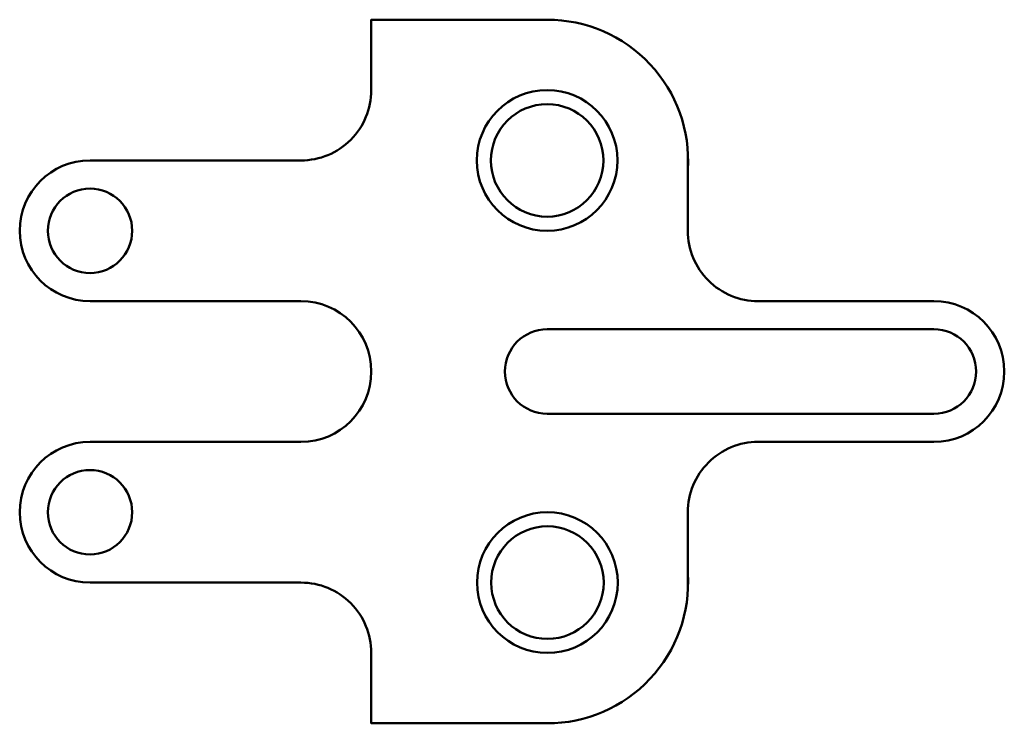
# Model space of a CAD drawing. Units: inches. Extents: x 1100 to 1240, y 1123 to 1223.
import ezdxf

# ---------------------------------------------------------------- set-up
doc = ezdxf.new("R2010")
doc.units = ezdxf.units.IN
doc.header["$MEASUREMENT"] = 0
doc.layers.add('M-OUTL', color=7, linetype='Continuous', lineweight=50)

# ---------------------------------------------------------------- blocks, each defined once
blk = doc.blocks.new('HOLE-CBORE-D16')
for radius in [10, 8]:
    blk.add_circle((1174.65, 1203.2, 23), radius)

msp = doc.modelspace()

# ---------------------------------------------------------------- linework, layer by layer
at = {"layer": 'M-OUTL', "extrusion": (0, 1, 0)}
msp.add_line((1109.65, 1203.2), (1124.65, 1203.2), dxfattribs=at)
at = {"layer": 'M-OUTL'}
for p, q in [((1129.65, 1203.2), (1139.65, 1203.2)), ((1194.65, 1203.2), (1194.69, 1203.2)), ((1139.65, 1183.2), (1109.65, 1183.2)), ((1174.65, 1179.2), (1229.65, 1179.2)), ((1174.65, 1167.2), (1229.65, 1167.2)), ((1139.65, 1163.2), (1109.65, 1163.2))]:
    msp.add_line(p, q, dxfattribs=at)
for points in [[(1109.65, 1203.2), (1139.65, 1203.2, 0.414214), (1149.65, 1213.2), (1149.65, 1223.2), (1174.69, 1223.2)], [(1194.65, 1204.49), (1194.65, 1193.2, 0.414214), (1204.65, 1183.2), (1229.65, 1183.2, -1), (1229.65, 1163.2)], [(1194.65, 1141.92), (1194.65, 1153.2, -0.414214), (1204.65, 1163.2), (1229.65, 1163.2)], [(1109.65, 1143.2), (1139.65, 1143.2, -0.414214), (1149.65, 1133.2), (1149.65, 1123.2), (1174.69, 1123.2)]]:
    msp.add_lwpolyline(points, format="xyb", dxfattribs=at)
at = {"layer": 'M-OUTL', "extrusion": (0, 1, 0)}
msp.add_circle((-1124.65, 11.5, 1203.2), 7.5, dxfattribs=at)
at = {"layer": 'M-OUTL'}
for centre in [(1109.65, 1193.2, 23), (1109.65, 1153.2)]:
    msp.add_circle(centre, 6, dxfattribs=at)
for centre, radius, start, end in [((1174.69, 1203.2), 20, 356.3118, 90.1187), ((1109.65, 1193.2), 10, 90, 270), ((1139.65, 1173.2), 10, 270, 90), ((1174.65, 1173.2), 6, 90, 270), ((1229.65, 1173.2), 6, 270, 90), ((1109.65, 1153.2), 10, 90, 270), ((1174.69, 1143.2), 20, 269.8813, 3.6882)]:
    msp.add_arc(centre, radius, start, end, dxfattribs=at)

# ---------------------------------------------------------------- block references
for p in [(0, 0), (0.04, -60)]:
    msp.add_blockref('HOLE-CBORE-D16', p, dxfattribs=at)

doc.saveas('drawing.dxf')
